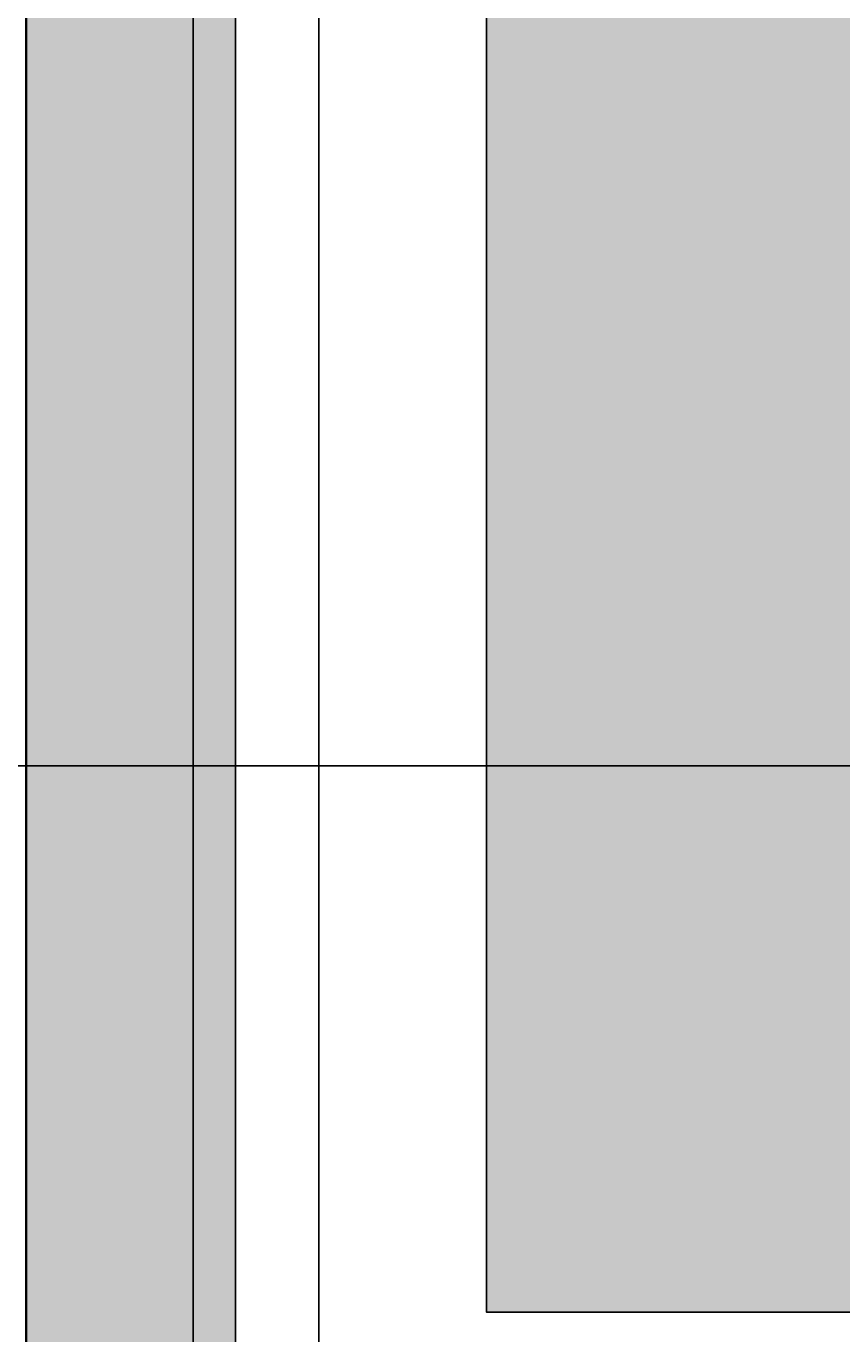
# Model space of a CAD drawing. Units: inches. Extents: x -301 to 715, y -607 to 364.
# Tile 21 of 141: x -35 to -16, y -453 to -422. Entities that reach past the tile are written whole.
import ezdxf

# ---------------------------------------------------------------- set-up
doc = ezdxf.new("R2010")
doc.units = ezdxf.units.IN
doc.header["$MEASUREMENT"] = 0
for name, color, linetype, lineweight in [('A-ANNO-DIMS', 2, 'Continuous', 18), ('A-DOOR', 4, 'Continuous', 25), ('A-SECT', 1, 'Continuous', 35), ('A-SECT-PATT', 8, 'Continuous', 13)]:
    doc.layers.add(name, color=color, linetype=linetype, lineweight=lineweight)
doc.styles.get("Standard").update_dxf_attribs({"font": 'arial.ttf'})
doc.dimstyles.get("Standard").update_dxf_attribs({"dimtxt": 0.18, "dimasz": 0.18, "dimexe": 0.18, "dimexo": 0.0625, "dimgap": 0.09, "dimtad": 0, "dimtih": 1, "dimtoh": 1, "dimdec": 1, "dimzin": 0, "dimdsep": 46, "dimlunit": 4, "dimtxsty": 'Standard', "dimcen": 0.09, "dimclrd": 3, "dimclre": 4, "dimclrt": 6, "dimadec": 0, "dimazin": 0, "dimtfac": 1, "dimtdec": 1, "dimtofl": 0, "dimtmove": 0, "dimatfit": 3, "dimfxl": 1, "dimtfill": 2, "dimtfillclr": 51, "dimtolj": 1, "dimtzin": 0, "dimarcsym": 0})

# ---------------------------------------------------------------- blocks, each defined once
blk = doc.blocks.new('*U75')
blk.add_lwpolyline([(3.124, 0.013), (0.124, 0.013), (0.124, 72.013), (40.124, 72.013), (40.124, 0.013), (37.124, 0.013)])
for points in [[(37.124, 68.99), (37.124, 0.013), (3.124, 0.013), (3.124, 68.99)], [(33.124, 6.013), (33.124, 62.99), (7.124, 62.99), (7.124, 6.013)]]:
    blk.add_lwpolyline(points, close=True)
blk = doc.blocks.new('*D187')
at = {"layer": 'A-ANNO-DIMS', "color": 4, "lineweight": -2, "transparency": 16777216}
for p, q in [((139.674, -385.477), (-266.112, -385.477)), ((143.155, -439.477), (-266.112, -439.477))]:
    blk.add_line(p, q, dxfattribs=at)
at = {"layer": 'A-ANNO-DIMS', "color": 3, "lineweight": -2, "transparency": 16777216}
for p, q in [((-265.932, -385.657), (-265.932, -412.296)), ((-265.932, -439.297), (-265.932, -412.659))]:
    blk.add_line(p, q, dxfattribs=at)
at = {"layer": 'A-ANNO-DIMS', "color": 3, "transparency": 16777216}
for points in [[(-265.962, -385.657), (-265.902, -385.657), (-265.932, -385.477)], [(-265.962, -439.297), (-265.902, -439.297), (-265.932, -439.477)]]:
    blk.add_solid(points, dxfattribs=at)
at = {"layer": 'Defpoints', "color": 0, "transparency": 16777216}
for p in [(-265.932, -385.477), (139.737, -385.477), (143.218, -439.477)]:
    blk.add_point(p, dxfattribs=at)
at = {"layer": 'A-ANNO-DIMS', "color": 6, "transparency": 16777216, "insert": (-265.932, -412.477), "char_height": 0.18, "attachment_point": 5, "bg_fill": 1, "box_fill_scale": 1.25, "bg_fill_color": 51, "bg_fill_transparency": 0}
blk.add_mtext('\\A1;4\'-6"', dxfattribs=at)

msp = doc.modelspace()

# ---------------------------------------------------------------- hatches: boundary and pattern name
at = {"layer": 'A-SECT-PATT'}
h = msp.add_hatch(color=256, dxfattribs=at)
h.dxf.hatch_style = 1
h.paths.add_polyline_path([(-138.282, -385.477), (-138.282, -433.477), (-87.981, -433.477), (-87.981, -385.477)])
h.paths.add_polyline_path([(-92.981, -390.477), (-92.981, -428.477), (-133.282, -428.477), (-133.282, -390.477)], flags=16)
h.paths.add_polyline_path([(-35.282, -385.477), (-35.282, -463.477), (12.718, -463.477), (12.718, -385.477)])
h.paths.add_polyline_path([(-30.282, -390.477), (7.718, -390.477), (7.718, -458.477), (-30.282, -458.477)], flags=16)
h.paths.add_polyline_path([(48.468, -385.477), (48.468, -433.477), (98.468, -433.477), (98.468, -385.477)])
h.paths.add_polyline_path([(93.468, -390.477), (93.468, -428.477), (53.468, -428.477), (53.468, -390.477)], flags=16)
h = msp.add_hatch(color=256, dxfattribs=at)
h.dxf.hatch_style = 1
h.paths.add_polyline_path([(-24.297, -452.509), (1.703, -452.509), (1.703, -395.532), (-24.297, -395.532)])

# ---------------------------------------------------------------- linework, layer by layer
at = {"layer": 'A-DOOR'}
for points in [[(-35.282, -385.477), (12.718, -385.477), (12.718, -463.477), (-35.282, -463.477)], [(-30.282, -390.477), (7.718, -390.477), (7.718, -458.477), (-30.282, -458.477)]]:
    msp.add_lwpolyline(points, close=True, dxfattribs=at)
at = {"layer": 'A-SECT'}
msp.add_line((-35.282, -361.477), (-35.282, -463.477), dxfattribs=at)

# ---------------------------------------------------------------- block references
at = {"layer": 'A-DOOR'}
msp.add_blockref('*U75', (-31.421, -458.522), dxfattribs=at)

# ---------------------------------------------------------------- dimensions: what is measured, and where the dimension line sits
at = {"layer": 'A-ANNO-DIMS'}
dim = msp.add_linear_dim(base=(-265.932, -385.477), p1=(143.218, -439.477), p2=(139.737, -385.477), angle=90, dimstyle='Standard', override={"dimdec": 1, "dimlfac": 1, "dimrnd": 0, "dimzin": 1, "dimdsep": 46, "dimlunit": 4, "dimfrac": 2}, dxfattribs=at)
dim.commit()
dim.dimension.update_dxf_attribs({"geometry": '*D187', "text_midpoint": (-265.932, -412.477)})

doc.saveas('drawing.dxf')
